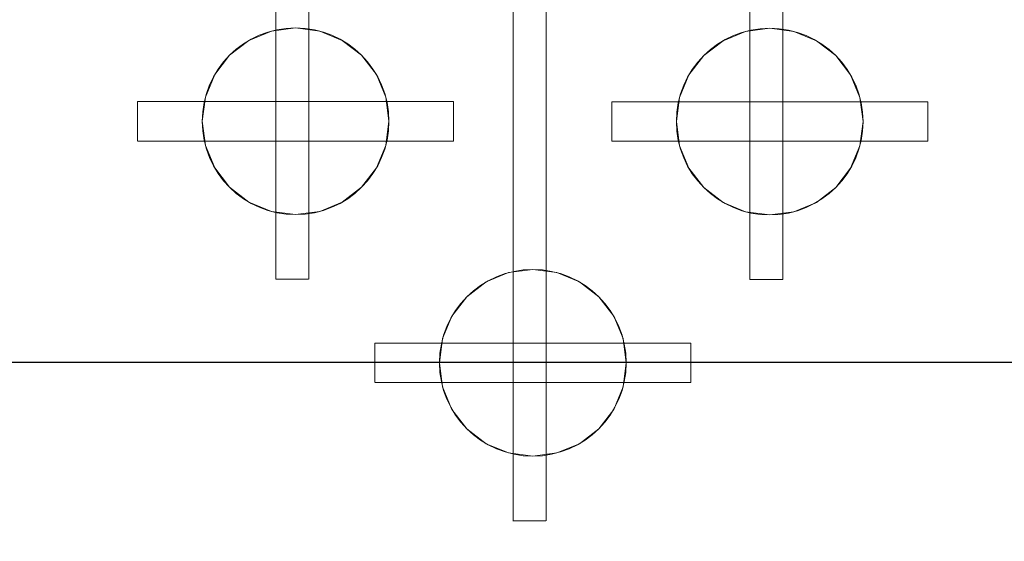
# Model space of a CAD drawing. Units: inches. Extents: x 2696 to 3240, y 1564 to 2310.
# Tile 19 of 76: x 2783.067 to 2792.41, y 1900.004 to 1904.955. Entities that reach past the tile are written whole.
import ezdxf

# ---------------------------------------------------------------- set-up
doc = ezdxf.new("R2010")
doc.units = ezdxf.units.IN
for name, color, linetype, lineweight in [('A-ANNO-DIMS', 3, 'Continuous', 18), ('A-FLOR-FIXT', 8, 'Continuous', 18), ('A-FURN', 251, 'Continuous', 13)]:
    doc.layers.add(name, color=color, linetype=linetype, lineweight=lineweight)
doc.layers.add('FURNITURE', color=250, linetype='Continuous')
doc.styles.add('TIMES NEW', font='times.ttf')
doc.dimstyles.new('Siddhuu', dxfattribs={"dimtxt": 6, "dimasz": 2.5, "dimexe": 1.25, "dimexo": 0.625, "dimtad": 1, "dimdec": 1, "dimlunit": 4, "dimtxsty": 'TIMES NEW', "dimcen": 2.5, "dimclrd": 256, "dimclre": 1, "dimclrt": 7, "dimadec": 0, "dimazin": 0, "dimtfac": 1, "dimtdec": 1, "dimtmove": 0, "dimatfit": 3, "dimfxl": 1, "dimtolj": 1, "dimlwd": -1, "dimarcsym": 0})

# ---------------------------------------------------------------- blocks, each defined once
blk = doc.blocks.new('A$C1af1f523')
at = {"layer": 'A-FURN'}
for p, q in [((-2.9003, 3.9351), (-2.9003, 0.9365)), ((-2.9003, 3.9351, 0.5), (-2.9003, 0.9365, 0.5)), ((-2.9003, 3.9351), (-2.9003, 3.9351, 0.5)), ((-2.5253, 3.9351), (-2.9003, 3.9351)), ((-2.5253, 3.9351, 0.5), (-2.9003, 3.9351, 0.5)), ((-2.5253, 3.9351), (-2.5253, 0.9365)), ((-2.5253, 3.9351, 0.5), (-2.5253, 0.9365, 0.5)), ((-2.5253, 3.9351), (-2.5253, 3.9351, 0.5)), ((-2.9421, 3.2913), (-2.9421, 3.2913, 0.5)), ((-2.7128, 3.3215), (-2.7128, 3.3215, 0.5)), ((-2.4835, 3.2913), (-2.4835, 3.2913, 0.5)), ((-3.1558, 3.2028), (-3.1558, 3.2028, 0.5)), ((-2.2698, 3.2028), (-2.2698, 3.2028, 0.5)), ((-3.3393, 3.062), (-3.3393, 3.062, 0.5)), ((-2.0863, 3.062), (-2.0863, 3.062, 0.5)), ((-3.4801, 2.8785), (-3.4801, 2.8785, 0.5)), ((-1.9455, 2.8785), (-1.9455, 2.8785, 0.5)), ((-3.5686, 2.6648), (-3.5686, 2.6648, 0.5)), ((-1.857, 2.6648), (-1.857, 2.6648, 0.5)), ((0, 2.5605), (-4.2116, 2.5605)), ((0, 2.5605, 0.5), (-4.2116, 2.5605, 0.5)), ((-4.2116, 2.5605), (-4.2116, 2.5605, 0.5)), ((-4.2116, 2.5594), (-4.2116, 2.248)), ((-4.2116, 2.5594, 0.5), (-4.2116, 2.248, 0.5)), ((-4.2116, 2.5594), (-4.2116, 2.5594, 0.5)), ((-3.5988, 2.4355), (-3.5988, 2.4355, 0.5)), ((-1.8268, 2.4355), (-1.8268, 2.4355, 0.5)), ((0, 2.248), (-4.2116, 2.248)), ((0, 2.248, 0.5), (-4.2116, 2.248, 0.5)), ((-4.2116, 2.248), (-4.2116, 2.248, 0.5)), ((-4.2116, 2.248), (-4.2116, 2.2469)), ((-4.2116, 2.248, 0.5), (-4.2116, 2.2469, 0.5)), ((-4.2116, 2.2469), (-4.2116, 2.2469, 0.5)), ((-3.5686, 2.2061), (-3.5686, 2.2061, 0.5)), ((-1.857, 2.2061), (-1.857, 2.2061, 0.5)), ((-3.4801, 1.9924), (-3.4801, 1.9924, 0.5)), ((-1.9455, 1.9924), (-1.9455, 1.9924, 0.5)), ((-3.3393, 1.8089), (-3.3393, 1.8089, 0.5)), ((-2.0863, 1.8089), (-2.0863, 1.8089, 0.5)), ((-4.8156, 1.6871), (-5.1906, 1.6871)), ((-4.8156, 1.6871, 0.5), (-5.1906, 1.6871, 0.5)), ((-5.1906, 1.6871), (-5.1906, 1.6871, 0.5)), ((-5.1906, 1.6871), (-5.1901, -1.3115)), ((-5.1906, 1.6871, 0.5), (-5.1901, -1.3115, 0.5)), ((-4.8156, 1.6871), (-4.8156, 1.6871, 0.5)), ((-4.8156, 1.6871), (-4.8151, -1.3115)), ((-4.8156, 1.6871, 0.5), (-4.8151, -1.3115, 0.5)), ((-3.1558, 1.6681), (-3.1558, 1.6681, 0.5)), ((-2.2698, 1.6681), (-2.2698, 1.6681, 0.5)), ((-2.9421, 1.5796), (-2.9421, 1.5796, 0.5)), ((-2.7128, 1.5494), (-2.7128, 1.5494, 0.5)), ((-2.4835, 1.5796), (-2.4835, 1.5796, 0.5)), ((-5.232, 1.0433), (-5.232, 1.0433, 0.5)), ((-5.0026, 1.0735), (-5.0026, 1.0735, 0.5)), ((-4.7733, 1.0433), (-4.7733, 1.0433, 0.5)), ((-5.4457, 0.9548), (-5.4457, 0.9548, 0.5)), ((-4.5596, 0.9548), (-4.5596, 0.9548, 0.5)), ((-2.9003, 0.9365), (-2.9003, 0.9365, 0.5)), ((-2.5253, 0.9365), (-2.8979, 0.9365)), ((-2.5253, 0.9365, 0.5), (-2.8979, 0.9365, 0.5)), ((-2.8979, 0.9365), (-2.8979, 0.9365, 0.5)), ((-2.5253, 0.9365), (-2.5253, 0.9365, 0.5)), ((-5.6292, 0.814), (-5.6292, 0.814, 0.5)), ((-4.3761, 0.814), (-4.3761, 0.814, 0.5)), ((-5.77, 0.6305), (-5.77, 0.6305, 0.5)), ((-4.2353, 0.6305), (-4.2353, 0.6305, 0.5)), ((-5.8585, 0.4168), (-5.8585, 0.4168, 0.5)), ((-4.1468, 0.4168), (-4.1468, 0.4168, 0.5)), ((0, 0.3125), (-6.5015, 0.3125)), ((0, 0.3125, 0.5), (-6.5015, 0.3125, 0.5)), ((-6.5015, 0.3125), (-6.5015, 0.3125, 0.5)), ((-6.5015, 0.3114), (-6.5015, 0)), ((-6.5015, 0.3114, 0.5), (-6.5015, 0, 0.5)), ((-6.5015, 0.3114), (-6.5015, 0.3114, 0.5)), ((-5.8887, 0.1875), (-5.8887, 0.1875, 0.5)), ((-4.1166, 0.1875), (-4.1166, 0.1875, 0.5)), ((0, 0), (-6.5015, 0)), ((0, 0, 0.5), (-6.5015, 0, 0.5)), ((-6.5015, 0), (-6.5015, 0, 0.5)), ((-6.5015, 0), (-6.5015, -0.0011)), ((-6.5015, 0, 0.5), (-6.5015, -0.0011, 0.5)), ((-6.5015, -0.0011), (-6.5015, -0.0011, 0.5)), ((-5.8585, -0.0418), (-5.8585, -0.0418, 0.5)), ((-4.1468, -0.0418), (-4.1468, -0.0418, 0.5)), ((-5.77, -0.2555), (-5.77, -0.2555, 0.5)), ((-4.2353, -0.2555), (-4.2353, -0.2555, 0.5)), ((-5.6292, -0.439), (-5.6292, -0.439, 0.5)), ((-4.3761, -0.439), (-4.3761, -0.439, 0.5)), ((-5.4457, -0.5798), (-5.4457, -0.5798, 0.5)), ((-4.5596, -0.5798), (-4.5596, -0.5798, 0.5)), ((-2.898, -0.5642), (-2.898, -3.5628)), ((-2.898, -0.5642, 0.5), (-2.898, -3.5628, 0.5)), ((-2.898, -0.5642), (-2.898, -0.5642, 0.5)), ((-2.523, -0.5642), (-2.898, -0.5642)), ((-2.523, -0.5642, 0.5), (-2.898, -0.5642, 0.5)), ((-2.523, -0.5642), (-2.523, -3.5628)), ((-2.523, -0.5642, 0.5), (-2.523, -3.5628, 0.5)), ((-2.523, -0.5642), (-2.523, -0.5642, 0.5)), ((-5.232, -0.6683), (-5.232, -0.6683, 0.5)), ((-5.0026, -0.6985), (-5.0026, -0.6985, 0.5)), ((-4.7733, -0.6683), (-4.7733, -0.6683, 0.5)), ((-2.9398, -1.208), (-2.9398, -1.208, 0.5)), ((-2.7105, -1.1778), (-2.7105, -1.1778, 0.5)), ((-2.4812, -1.208), (-2.4812, -1.208, 0.5)), ((-3.1535, -1.2965), (-3.1535, -1.2965, 0.5)), ((-2.2675, -1.2965), (-2.2675, -1.2965, 0.5)), ((-5.1901, -1.3115), (-5.1901, -1.3115, 0.5)), ((-4.8151, -1.3115), (-5.1878, -1.3115)), ((-4.8151, -1.3115, 0.5), (-5.1878, -1.3115, 0.5)), ((-5.1878, -1.3115), (-5.1878, -1.3115, 0.5)), ((-4.8151, -1.3115), (-4.8151, -1.3115, 0.5)), ((-3.337, -1.4373), (-3.337, -1.4373, 0.5)), ((-2.084, -1.4373), (-2.084, -1.4373, 0.5)), ((-3.4778, -1.6208), (-3.4778, -1.6208, 0.5)), ((-1.9432, -1.6208), (-1.9432, -1.6208, 0.5)), ((-3.5664, -1.8345), (-3.5664, -1.8345, 0.5)), ((-1.8547, -1.8345), (-1.8547, -1.8345, 0.5)), ((0, -1.9388), (-4.2094, -1.9388)), ((0, -1.9388, 0.5), (-4.2094, -1.9388, 0.5)), ((-4.2094, -1.9388), (-4.2094, -1.9388, 0.5)), ((-4.2094, -1.9399), (-4.2094, -2.2513)), ((-4.2094, -1.9399, 0.5), (-4.2094, -2.2513, 0.5)), ((-4.2094, -1.9399), (-4.2094, -1.9399, 0.5)), ((-3.5965, -2.0638), (-3.5965, -2.0638, 0.5)), ((-1.8245, -2.0638), (-1.8245, -2.0638, 0.5)), ((0, -2.2513), (-4.2094, -2.2513)), ((0, -2.2513, 0.5), (-4.2094, -2.2513, 0.5)), ((-4.2094, -2.2513), (-4.2094, -2.2513, 0.5)), ((-4.2094, -2.2513), (-4.2094, -2.2524)), ((-4.2094, -2.2513, 0.5), (-4.2094, -2.2524, 0.5)), ((-4.2094, -2.2524), (-4.2094, -2.2524, 0.5)), ((-3.5664, -2.2931), (-3.5664, -2.2931, 0.5)), ((-1.8547, -2.2931), (-1.8547, -2.2931, 0.5)), ((-3.4778, -2.5068), (-3.4778, -2.5068, 0.5)), ((-1.9432, -2.5068), (-1.9432, -2.5068, 0.5)), ((-3.337, -2.6903), (-3.337, -2.6903, 0.5)), ((-2.084, -2.6903), (-2.084, -2.6903, 0.5)), ((-3.1535, -2.8311), (-3.1535, -2.8311, 0.5)), ((-2.2675, -2.8311), (-2.2675, -2.8311, 0.5)), ((-2.9398, -2.9196), (-2.9398, -2.9196, 0.5)), ((-2.7105, -2.9498), (-2.7105, -2.9498, 0.5)), ((-2.4812, -2.9196), (-2.4812, -2.9196, 0.5)), ((-2.898, -3.5628), (-2.898, -3.5628, 0.5)), ((-2.523, -3.5628), (-2.8956, -3.5628)), ((-2.523, -3.5628, 0.5), (-2.8956, -3.5628, 0.5)), ((-2.8956, -3.5628), (-2.8956, -3.5628, 0.5)), ((-2.523, -3.5628), (-2.523, -3.5628, 0.5))]:
    blk.add_line(p, q, dxfattribs=at)
for centre in [(-2.7128, 2.4355), (-2.7128, 2.4355, 0.5), (-5.0026, 0.1875), (-5.0026, 0.1875, 0.5), (-2.7105, -2.0638), (-2.7105, -2.0638, 0.5)]:
    blk.add_circle(centre, 0.886, dxfattribs=at)
at = {"layer": 'FURNITURE'}
for p, q in [((0, 2.5605), (0, 2.5605, 0.5)), ((0, 2.248), (0, 2.248, 0.5)), ((0, 0.3125), (0, 0.3125, 0.5)), ((0, 0), (0, 0, 0.5)), ((0, -1.9388), (0, -1.9388, 0.5)), ((0, -2.2513), (0, -2.2513, 0.5))]:
    blk.add_line(p, q, dxfattribs=at)
at = {"layer": 'A-FURN'}
mesh = blk.add_polyface(dxfattribs=at)
corners = [(-2.9003, 0.9365, 0.5), (-2.9003, 3.9351), (-2.9003, 0.9365), (-2.9003, 3.9351, 0.5)]
mesh.append_faces([[corners[k] for k in face] for face in [(2, 1, 0), (3, 0, 1)]], dxfattribs={"vtx1": -1})
mesh = blk.add_polyface(dxfattribs=at)
corners = [(-2.5253, 3.9351, 0.5), (-2.9003, 3.9351), (-2.9003, 3.9351, 0.5), (-2.5253, 3.9351)]
mesh.append_faces([[corners[k] for k in face] for face in [(2, 1, 0), (3, 0, 1)]], dxfattribs={"vtx1": -1})
mesh = blk.add_polyface(dxfattribs=at)
corners = [(-2.5253, 0.9365, 0.5), (-2.5253, 3.9351), (-2.5253, 0.9365), (-2.5253, 3.9351, 0.5)]
mesh.append_faces([[corners[k] for k in face] for face in [(2, 1, 0), (3, 0, 1)]], dxfattribs={"vtx1": -1})
mesh = blk.add_polyface(dxfattribs=at)
corners = [(-2.9421, 3.2913), (-3.1558, 3.2028, 0.5), (-3.1558, 3.2028), (-2.9421, 3.2913, 0.5)]
mesh.append_faces([[corners[k] for k in face] for face in [(2, 1, 0), (3, 0, 1)]], dxfattribs={"vtx1": -1})
mesh = blk.add_polyface(dxfattribs=at)
corners = [(-2.7128, 3.3215), (-2.9421, 3.2913, 0.5), (-2.9421, 3.2913), (-2.7128, 3.3215, 0.5)]
mesh.append_faces([[corners[k] for k in face] for face in [(2, 1, 0), (3, 0, 1)]], dxfattribs={"vtx1": -1})
mesh = blk.add_polyface(dxfattribs=at)
corners = [(-2.4835, 3.2913), (-2.7128, 3.3215, 0.5), (-2.7128, 3.3215), (-2.4835, 3.2913, 0.5)]
mesh.append_faces([[corners[k] for k in face] for face in [(2, 1, 0), (3, 0, 1)]], dxfattribs={"vtx1": -1})
mesh = blk.add_polyface(dxfattribs=at)
corners = [(-2.2698, 3.2028), (-2.4835, 3.2913, 0.5), (-2.4835, 3.2913), (-2.2698, 3.2028, 0.5)]
mesh.append_faces([[corners[k] for k in face] for face in [(2, 1, 0), (3, 0, 1)]], dxfattribs={"vtx1": -1})
mesh = blk.add_polyface(dxfattribs=at)
corners = [(-3.1558, 3.2028), (-3.3393, 3.062, 0.5), (-3.3393, 3.062), (-3.1558, 3.2028, 0.5)]
mesh.append_faces([[corners[k] for k in face] for face in [(2, 1, 0), (3, 0, 1)]], dxfattribs={"vtx1": -1})
mesh = blk.add_polyface(dxfattribs=at)
corners = [(-2.0863, 3.062), (-2.2698, 3.2028, 0.5), (-2.2698, 3.2028), (-2.0863, 3.062, 0.5)]
mesh.append_faces([[corners[k] for k in face] for face in [(2, 1, 0), (3, 0, 1)]], dxfattribs={"vtx1": -1})
mesh = blk.add_polyface(dxfattribs=at)
corners = [(-3.3393, 3.062, 0.5), (-3.4801, 2.8785), (-3.3393, 3.062), (-3.4801, 2.8785, 0.5)]
mesh.append_faces([[corners[k] for k in face] for face in [(2, 1, 0), (3, 0, 1)]], dxfattribs={"vtx1": -1})
mesh = blk.add_polyface(dxfattribs=at)
corners = [(-1.9455, 2.8785, 0.5), (-2.0863, 3.062), (-1.9455, 2.8785), (-2.0863, 3.062, 0.5)]
mesh.append_faces([[corners[k] for k in face] for face in [(2, 1, 0), (3, 0, 1)]], dxfattribs={"vtx1": -1})
mesh = blk.add_polyface(dxfattribs=at)
corners = [(-3.4801, 2.8785, 0.5), (-3.5686, 2.6648), (-3.4801, 2.8785), (-3.5686, 2.6648, 0.5)]
mesh.append_faces([[corners[k] for k in face] for face in [(2, 1, 0), (3, 0, 1)]], dxfattribs={"vtx1": -1})
mesh = blk.add_polyface(dxfattribs=at)
corners = [(-1.857, 2.6648, 0.5), (-1.9455, 2.8785), (-1.857, 2.6648), (-1.9455, 2.8785, 0.5)]
mesh.append_faces([[corners[k] for k in face] for face in [(2, 1, 0), (3, 0, 1)]], dxfattribs={"vtx1": -1})
mesh = blk.add_polyface(dxfattribs=at)
corners = [(-3.5686, 2.6648, 0.5), (-3.5988, 2.4355), (-3.5686, 2.6648), (-3.5988, 2.4355, 0.5)]
mesh.append_faces([[corners[k] for k in face] for face in [(2, 1, 0), (3, 0, 1)]], dxfattribs={"vtx1": -1})
mesh = blk.add_polyface(dxfattribs=at)
corners = [(-1.8268, 2.4355, 0.5), (-1.857, 2.6648), (-1.8268, 2.4355), (-1.857, 2.6648, 0.5)]
mesh.append_faces([[corners[k] for k in face] for face in [(2, 1, 0), (3, 0, 1)]], dxfattribs={"vtx1": -1})
mesh = blk.add_polyface(dxfattribs=at)
corners = [(0, 2.5605, 0.5), (-4.2116, 2.5605), (-4.2116, 2.5605, 0.5), (0, 2.5605)]
mesh.append_faces([[corners[k] for k in face] for face in [(2, 1, 0), (3, 0, 1)]], dxfattribs={"vtx1": -1})
mesh = blk.add_polyface(dxfattribs=at)
corners = [(-4.2116, 2.2469, 0.5), (-4.2116, 2.248), (-4.2116, 2.2469), (-4.2116, 2.5594), (-4.2116, 2.5594, 0.5), (-4.2116, 2.248, 0.5)]
mesh.append_faces([[corners[k] for k in face] for face in [(3, 0, 1), (4, 0, 3)]], dxfattribs={"vtx0": -1, "vtx1": -1})
mesh.append_faces([[corners[k] for k in face] for face in [(2, 1, 0), (5, 0, 4)]], dxfattribs={"vtx1": -1})
mesh = blk.add_polyface(dxfattribs=at)
corners = [(-3.5988, 2.4355, 0.5), (-3.5686, 2.2061), (-3.5988, 2.4355), (-3.5686, 2.2061, 0.5)]
mesh.append_faces([[corners[k] for k in face] for face in [(2, 1, 0), (3, 0, 1)]], dxfattribs={"vtx1": -1})
mesh = blk.add_polyface(dxfattribs=at)
corners = [(-1.857, 2.2061, 0.5), (-1.8268, 2.4355), (-1.857, 2.2061), (-1.8268, 2.4355, 0.5)]
mesh.append_faces([[corners[k] for k in face] for face in [(2, 1, 0), (3, 0, 1)]], dxfattribs={"vtx1": -1})
mesh = blk.add_polyface(dxfattribs=at)
corners = [(0, 2.248, 0.5), (-4.2116, 2.248), (-4.2116, 2.248, 0.5), (0, 2.248)]
mesh.append_faces([[corners[k] for k in face] for face in [(2, 1, 0), (3, 0, 1)]], dxfattribs={"vtx1": -1})
mesh = blk.add_polyface(dxfattribs=at)
corners = [(-3.5686, 2.2061, 0.5), (-3.4801, 1.9924), (-3.5686, 2.2061), (-3.4801, 1.9924, 0.5)]
mesh.append_faces([[corners[k] for k in face] for face in [(2, 1, 0), (3, 0, 1)]], dxfattribs={"vtx1": -1})
mesh = blk.add_polyface(dxfattribs=at)
corners = [(-1.9455, 1.9924, 0.5), (-1.857, 2.2061), (-1.9455, 1.9924), (-1.857, 2.2061, 0.5)]
mesh.append_faces([[corners[k] for k in face] for face in [(2, 1, 0), (3, 0, 1)]], dxfattribs={"vtx1": -1})
mesh = blk.add_polyface(dxfattribs=at)
corners = [(-3.4801, 1.9924, 0.5), (-3.3393, 1.8089), (-3.4801, 1.9924), (-3.3393, 1.8089, 0.5)]
mesh.append_faces([[corners[k] for k in face] for face in [(2, 1, 0), (3, 0, 1)]], dxfattribs={"vtx1": -1})
mesh = blk.add_polyface(dxfattribs=at)
corners = [(-2.0863, 1.8089, 0.5), (-1.9455, 1.9924), (-2.0863, 1.8089), (-1.9455, 1.9924, 0.5)]
mesh.append_faces([[corners[k] for k in face] for face in [(2, 1, 0), (3, 0, 1)]], dxfattribs={"vtx1": -1})
mesh = blk.add_polyface(dxfattribs=at)
corners = [(-3.1558, 1.6681, 0.5), (-3.3393, 1.8089), (-3.3393, 1.8089, 0.5), (-3.1558, 1.6681)]
mesh.append_faces([[corners[k] for k in face] for face in [(2, 1, 0), (3, 0, 1)]], dxfattribs={"vtx1": -1})
mesh = blk.add_polyface(dxfattribs=at)
corners = [(-2.0863, 1.8089, 0.5), (-2.2698, 1.6681), (-2.2698, 1.6681, 0.5), (-2.0863, 1.8089)]
mesh.append_faces([[corners[k] for k in face] for face in [(2, 1, 0), (3, 0, 1)]], dxfattribs={"vtx1": -1})
mesh = blk.add_polyface(dxfattribs=at)
corners = [(-4.8156, 1.6871, 0.5), (-5.1906, 1.6871), (-5.1906, 1.6871, 0.5), (-4.8156, 1.6871)]
mesh.append_faces([[corners[k] for k in face] for face in [(2, 1, 0), (3, 0, 1)]], dxfattribs={"vtx1": -1})
mesh = blk.add_polyface(dxfattribs=at)
corners = [(-5.1901, -1.3115, 0.5), (-5.1906, 1.6871), (-5.1901, -1.3115), (-5.1906, 1.6871, 0.5)]
mesh.append_faces([[corners[k] for k in face] for face in [(2, 1, 0), (3, 0, 1)]], dxfattribs={"vtx1": -1})
mesh = blk.add_polyface(dxfattribs=at)
corners = [(-4.8151, -1.3115, 0.5), (-4.8156, 1.6871), (-4.8151, -1.3115), (-4.8156, 1.6871, 0.5)]
mesh.append_faces([[corners[k] for k in face] for face in [(2, 1, 0), (3, 0, 1)]], dxfattribs={"vtx1": -1})
mesh = blk.add_polyface(dxfattribs=at)
corners = [(-2.9421, 1.5796, 0.5), (-3.1558, 1.6681), (-3.1558, 1.6681, 0.5), (-2.9421, 1.5796)]
mesh.append_faces([[corners[k] for k in face] for face in [(2, 1, 0), (3, 0, 1)]], dxfattribs={"vtx1": -1})
mesh = blk.add_polyface(dxfattribs=at)
corners = [(-2.2698, 1.6681, 0.5), (-2.4835, 1.5796), (-2.4835, 1.5796, 0.5), (-2.2698, 1.6681)]
mesh.append_faces([[corners[k] for k in face] for face in [(2, 1, 0), (3, 0, 1)]], dxfattribs={"vtx1": -1})
mesh = blk.add_polyface(dxfattribs=at)
corners = [(-2.7128, 1.5494, 0.5), (-2.9421, 1.5796), (-2.9421, 1.5796, 0.5), (-2.7128, 1.5494)]
mesh.append_faces([[corners[k] for k in face] for face in [(2, 1, 0), (3, 0, 1)]], dxfattribs={"vtx1": -1})
mesh = blk.add_polyface(dxfattribs=at)
corners = [(-2.4835, 1.5796, 0.5), (-2.7128, 1.5494), (-2.7128, 1.5494, 0.5), (-2.4835, 1.5796)]
mesh.append_faces([[corners[k] for k in face] for face in [(2, 1, 0), (3, 0, 1)]], dxfattribs={"vtx1": -1})
mesh = blk.add_polyface(dxfattribs=at)
corners = [(-5.232, 1.0433), (-5.4457, 0.9548, 0.5), (-5.4457, 0.9548), (-5.232, 1.0433, 0.5)]
mesh.append_faces([[corners[k] for k in face] for face in [(2, 1, 0), (3, 0, 1)]], dxfattribs={"vtx1": -1})
mesh = blk.add_polyface(dxfattribs=at)
corners = [(-5.0026, 1.0735), (-5.232, 1.0433, 0.5), (-5.232, 1.0433), (-5.0026, 1.0735, 0.5)]
mesh.append_faces([[corners[k] for k in face] for face in [(2, 1, 0), (3, 0, 1)]], dxfattribs={"vtx1": -1})
mesh = blk.add_polyface(dxfattribs=at)
corners = [(-4.7733, 1.0433), (-5.0026, 1.0735, 0.5), (-5.0026, 1.0735), (-4.7733, 1.0433, 0.5)]
mesh.append_faces([[corners[k] for k in face] for face in [(2, 1, 0), (3, 0, 1)]], dxfattribs={"vtx1": -1})
mesh = blk.add_polyface(dxfattribs=at)
corners = [(-4.5596, 0.9548), (-4.7733, 1.0433, 0.5), (-4.7733, 1.0433), (-4.5596, 0.9548, 0.5)]
mesh.append_faces([[corners[k] for k in face] for face in [(2, 1, 0), (3, 0, 1)]], dxfattribs={"vtx1": -1})
mesh = blk.add_polyface(dxfattribs=at)
corners = [(-5.4457, 0.9548), (-5.6292, 0.814, 0.5), (-5.6292, 0.814), (-5.4457, 0.9548, 0.5)]
mesh.append_faces([[corners[k] for k in face] for face in [(2, 1, 0), (3, 0, 1)]], dxfattribs={"vtx1": -1})
mesh = blk.add_polyface(dxfattribs=at)
corners = [(-4.3761, 0.814), (-4.5596, 0.9548, 0.5), (-4.5596, 0.9548), (-4.3761, 0.814, 0.5)]
mesh.append_faces([[corners[k] for k in face] for face in [(2, 1, 0), (3, 0, 1)]], dxfattribs={"vtx1": -1})
mesh = blk.add_polyface(dxfattribs=at)
corners = [(-2.5253, 0.9365, 0.5), (-2.8979, 0.9365), (-2.8979, 0.9365, 0.5), (-2.5253, 0.9365)]
mesh.append_faces([[corners[k] for k in face] for face in [(2, 1, 0), (3, 0, 1)]], dxfattribs={"vtx1": -1})
mesh = blk.add_polyface(dxfattribs=at)
corners = [(-5.6292, 0.814, 0.5), (-5.77, 0.6305), (-5.6292, 0.814), (-5.77, 0.6305, 0.5)]
mesh.append_faces([[corners[k] for k in face] for face in [(2, 1, 0), (3, 0, 1)]], dxfattribs={"vtx1": -1})
mesh = blk.add_polyface(dxfattribs=at)
corners = [(-4.2353, 0.6305, 0.5), (-4.3761, 0.814), (-4.2353, 0.6305), (-4.3761, 0.814, 0.5)]
mesh.append_faces([[corners[k] for k in face] for face in [(2, 1, 0), (3, 0, 1)]], dxfattribs={"vtx1": -1})
mesh = blk.add_polyface(dxfattribs=at)
corners = [(-5.77, 0.6305, 0.5), (-5.8585, 0.4168), (-5.77, 0.6305), (-5.8585, 0.4168, 0.5)]
mesh.append_faces([[corners[k] for k in face] for face in [(2, 1, 0), (3, 0, 1)]], dxfattribs={"vtx1": -1})
mesh = blk.add_polyface(dxfattribs=at)
corners = [(-4.1468, 0.4168, 0.5), (-4.2353, 0.6305), (-4.1468, 0.4168), (-4.2353, 0.6305, 0.5)]
mesh.append_faces([[corners[k] for k in face] for face in [(2, 1, 0), (3, 0, 1)]], dxfattribs={"vtx1": -1})
mesh = blk.add_polyface(dxfattribs=at)
corners = [(-5.8585, 0.4168, 0.5), (-5.8887, 0.1875), (-5.8585, 0.4168), (-5.8887, 0.1875, 0.5)]
mesh.append_faces([[corners[k] for k in face] for face in [(2, 1, 0), (3, 0, 1)]], dxfattribs={"vtx1": -1})
mesh = blk.add_polyface(dxfattribs=at)
corners = [(-4.1166, 0.1875, 0.5), (-4.1468, 0.4168), (-4.1166, 0.1875), (-4.1468, 0.4168, 0.5)]
mesh.append_faces([[corners[k] for k in face] for face in [(2, 1, 0), (3, 0, 1)]], dxfattribs={"vtx1": -1})
mesh = blk.add_polyface(dxfattribs=at)
corners = [(0, 0.3125, 0.5), (-6.5015, 0.3125), (-6.5015, 0.3125, 0.5), (0, 0.3125)]
mesh.append_faces([[corners[k] for k in face] for face in [(2, 1, 0), (3, 0, 1)]], dxfattribs={"vtx1": -1})
mesh = blk.add_polyface(dxfattribs=at)
corners = [(-6.5015, -0.0011, 0.5), (-6.5015, 0), (-6.5015, -0.0011), (-6.5015, 0.3114), (-6.5015, 0.3114, 0.5), (-6.5015, 0, 0.5)]
mesh.append_faces([[corners[k] for k in face] for face in [(3, 0, 1), (4, 0, 3)]], dxfattribs={"vtx0": -1, "vtx1": -1})
mesh.append_faces([[corners[k] for k in face] for face in [(2, 1, 0), (5, 0, 4)]], dxfattribs={"vtx1": -1})
mesh = blk.add_polyface(dxfattribs=at)
corners = [(-5.8887, 0.1875, 0.5), (-5.8585, -0.0418), (-5.8887, 0.1875), (-5.8585, -0.0418, 0.5)]
mesh.append_faces([[corners[k] for k in face] for face in [(2, 1, 0), (3, 0, 1)]], dxfattribs={"vtx1": -1})
mesh = blk.add_polyface(dxfattribs=at)
corners = [(-4.1468, -0.0418, 0.5), (-4.1166, 0.1875), (-4.1468, -0.0418), (-4.1166, 0.1875, 0.5)]
mesh.append_faces([[corners[k] for k in face] for face in [(2, 1, 0), (3, 0, 1)]], dxfattribs={"vtx1": -1})
mesh = blk.add_polyface(dxfattribs=at)
corners = [(0, 0, 0.5), (-6.5015, 0), (-6.5015, 0, 0.5), (0, 0)]
mesh.append_faces([[corners[k] for k in face] for face in [(2, 1, 0), (3, 0, 1)]], dxfattribs={"vtx1": -1})
mesh = blk.add_polyface(dxfattribs=at)
corners = [(-5.8585, -0.0418, 0.5), (-5.77, -0.2555), (-5.8585, -0.0418), (-5.77, -0.2555, 0.5)]
mesh.append_faces([[corners[k] for k in face] for face in [(2, 1, 0), (3, 0, 1)]], dxfattribs={"vtx1": -1})
mesh = blk.add_polyface(dxfattribs=at)
corners = [(-4.2353, -0.2555, 0.5), (-4.1468, -0.0418), (-4.2353, -0.2555), (-4.1468, -0.0418, 0.5)]
mesh.append_faces([[corners[k] for k in face] for face in [(2, 1, 0), (3, 0, 1)]], dxfattribs={"vtx1": -1})
mesh = blk.add_polyface(dxfattribs=at)
corners = [(-5.77, -0.2555, 0.5), (-5.6292, -0.439), (-5.77, -0.2555), (-5.6292, -0.439, 0.5)]
mesh.append_faces([[corners[k] for k in face] for face in [(2, 1, 0), (3, 0, 1)]], dxfattribs={"vtx1": -1})
mesh = blk.add_polyface(dxfattribs=at)
corners = [(-4.3761, -0.439, 0.5), (-4.2353, -0.2555), (-4.3761, -0.439), (-4.2353, -0.2555, 0.5)]
mesh.append_faces([[corners[k] for k in face] for face in [(2, 1, 0), (3, 0, 1)]], dxfattribs={"vtx1": -1})
mesh = blk.add_polyface(dxfattribs=at)
corners = [(-5.4457, -0.5798, 0.5), (-5.6292, -0.439), (-5.6292, -0.439, 0.5), (-5.4457, -0.5798)]
mesh.append_faces([[corners[k] for k in face] for face in [(2, 1, 0), (3, 0, 1)]], dxfattribs={"vtx1": -1})
mesh = blk.add_polyface(dxfattribs=at)
corners = [(-4.3761, -0.439, 0.5), (-4.5596, -0.5798), (-4.5596, -0.5798, 0.5), (-4.3761, -0.439)]
mesh.append_faces([[corners[k] for k in face] for face in [(2, 1, 0), (3, 0, 1)]], dxfattribs={"vtx1": -1})
mesh = blk.add_polyface(dxfattribs=at)
corners = [(-5.232, -0.6683, 0.5), (-5.4457, -0.5798), (-5.4457, -0.5798, 0.5), (-5.232, -0.6683)]
mesh.append_faces([[corners[k] for k in face] for face in [(2, 1, 0), (3, 0, 1)]], dxfattribs={"vtx1": -1})
mesh = blk.add_polyface(dxfattribs=at)
corners = [(-4.5596, -0.5798, 0.5), (-4.7733, -0.6683), (-4.7733, -0.6683, 0.5), (-4.5596, -0.5798)]
mesh.append_faces([[corners[k] for k in face] for face in [(2, 1, 0), (3, 0, 1)]], dxfattribs={"vtx1": -1})
mesh = blk.add_polyface(dxfattribs=at)
corners = [(-2.898, -3.5628, 0.5), (-2.898, -0.5642), (-2.898, -3.5628), (-2.898, -0.5642, 0.5)]
mesh.append_faces([[corners[k] for k in face] for face in [(2, 1, 0), (3, 0, 1)]], dxfattribs={"vtx1": -1})
mesh = blk.add_polyface(dxfattribs=at)
corners = [(-2.523, -0.5642, 0.5), (-2.898, -0.5642), (-2.898, -0.5642, 0.5), (-2.523, -0.5642)]
mesh.append_faces([[corners[k] for k in face] for face in [(2, 1, 0), (3, 0, 1)]], dxfattribs={"vtx1": -1})
mesh = blk.add_polyface(dxfattribs=at)
corners = [(-2.523, -3.5628, 0.5), (-2.523, -0.5642), (-2.523, -3.5628), (-2.523, -0.5642, 0.5)]
mesh.append_faces([[corners[k] for k in face] for face in [(2, 1, 0), (3, 0, 1)]], dxfattribs={"vtx1": -1})
mesh = blk.add_polyface(dxfattribs=at)
corners = [(-5.0026, -0.6985, 0.5), (-5.232, -0.6683), (-5.232, -0.6683, 0.5), (-5.0026, -0.6985)]
mesh.append_faces([[corners[k] for k in face] for face in [(2, 1, 0), (3, 0, 1)]], dxfattribs={"vtx1": -1})
mesh = blk.add_polyface(dxfattribs=at)
corners = [(-4.7733, -0.6683, 0.5), (-5.0026, -0.6985), (-5.0026, -0.6985, 0.5), (-4.7733, -0.6683)]
mesh.append_faces([[corners[k] for k in face] for face in [(2, 1, 0), (3, 0, 1)]], dxfattribs={"vtx1": -1})
mesh = blk.add_polyface(dxfattribs=at)
corners = [(-2.9398, -1.208), (-3.1535, -1.2965, 0.5), (-3.1535, -1.2965), (-2.9398, -1.208, 0.5)]
mesh.append_faces([[corners[k] for k in face] for face in [(2, 1, 0), (3, 0, 1)]], dxfattribs={"vtx1": -1})
mesh = blk.add_polyface(dxfattribs=at)
corners = [(-2.7105, -1.1778), (-2.9398, -1.208, 0.5), (-2.9398, -1.208), (-2.7105, -1.1778, 0.5)]
mesh.append_faces([[corners[k] for k in face] for face in [(2, 1, 0), (3, 0, 1)]], dxfattribs={"vtx1": -1})
mesh = blk.add_polyface(dxfattribs=at)
corners = [(-2.4812, -1.208), (-2.7105, -1.1778, 0.5), (-2.7105, -1.1778), (-2.4812, -1.208, 0.5)]
mesh.append_faces([[corners[k] for k in face] for face in [(2, 1, 0), (3, 0, 1)]], dxfattribs={"vtx1": -1})
mesh = blk.add_polyface(dxfattribs=at)
corners = [(-2.2675, -1.2965), (-2.4812, -1.208, 0.5), (-2.4812, -1.208), (-2.2675, -1.2965, 0.5)]
mesh.append_faces([[corners[k] for k in face] for face in [(2, 1, 0), (3, 0, 1)]], dxfattribs={"vtx1": -1})
mesh = blk.add_polyface(dxfattribs=at)
corners = [(-3.1535, -1.2965), (-3.337, -1.4373, 0.5), (-3.337, -1.4373), (-3.1535, -1.2965, 0.5)]
mesh.append_faces([[corners[k] for k in face] for face in [(2, 1, 0), (3, 0, 1)]], dxfattribs={"vtx1": -1})
mesh = blk.add_polyface(dxfattribs=at)
corners = [(-2.084, -1.4373), (-2.2675, -1.2965, 0.5), (-2.2675, -1.2965), (-2.084, -1.4373, 0.5)]
mesh.append_faces([[corners[k] for k in face] for face in [(2, 1, 0), (3, 0, 1)]], dxfattribs={"vtx1": -1})
mesh = blk.add_polyface(dxfattribs=at)
corners = [(-4.8151, -1.3115, 0.5), (-5.1878, -1.3115), (-5.1878, -1.3115, 0.5), (-4.8151, -1.3115)]
mesh.append_faces([[corners[k] for k in face] for face in [(2, 1, 0), (3, 0, 1)]], dxfattribs={"vtx1": -1})
mesh = blk.add_polyface(dxfattribs=at)
corners = [(-3.337, -1.4373, 0.5), (-3.4778, -1.6208), (-3.337, -1.4373), (-3.4778, -1.6208, 0.5)]
mesh.append_faces([[corners[k] for k in face] for face in [(2, 1, 0), (3, 0, 1)]], dxfattribs={"vtx1": -1})
mesh = blk.add_polyface(dxfattribs=at)
corners = [(-1.9432, -1.6208, 0.5), (-2.084, -1.4373), (-1.9432, -1.6208), (-2.084, -1.4373, 0.5)]
mesh.append_faces([[corners[k] for k in face] for face in [(2, 1, 0), (3, 0, 1)]], dxfattribs={"vtx1": -1})
mesh = blk.add_polyface(dxfattribs=at)
corners = [(-3.4778, -1.6208, 0.5), (-3.5664, -1.8345), (-3.4778, -1.6208), (-3.5664, -1.8345, 0.5)]
mesh.append_faces([[corners[k] for k in face] for face in [(2, 1, 0), (3, 0, 1)]], dxfattribs={"vtx1": -1})
mesh = blk.add_polyface(dxfattribs=at)
corners = [(-1.8547, -1.8345, 0.5), (-1.9432, -1.6208), (-1.8547, -1.8345), (-1.9432, -1.6208, 0.5)]
mesh.append_faces([[corners[k] for k in face] for face in [(2, 1, 0), (3, 0, 1)]], dxfattribs={"vtx1": -1})
mesh = blk.add_polyface(dxfattribs=at)
corners = [(-3.5664, -1.8345, 0.5), (-3.5965, -2.0638), (-3.5664, -1.8345), (-3.5965, -2.0638, 0.5)]
mesh.append_faces([[corners[k] for k in face] for face in [(2, 1, 0), (3, 0, 1)]], dxfattribs={"vtx1": -1})
mesh = blk.add_polyface(dxfattribs=at)
corners = [(-1.8245, -2.0638, 0.5), (-1.8547, -1.8345), (-1.8245, -2.0638), (-1.8547, -1.8345, 0.5)]
mesh.append_faces([[corners[k] for k in face] for face in [(2, 1, 0), (3, 0, 1)]], dxfattribs={"vtx1": -1})
mesh = blk.add_polyface(dxfattribs=at)
corners = [(0, -1.9388, 0.5), (-4.2094, -1.9388), (-4.2094, -1.9388, 0.5), (0, -1.9388)]
mesh.append_faces([[corners[k] for k in face] for face in [(2, 1, 0), (3, 0, 1)]], dxfattribs={"vtx1": -1})
mesh = blk.add_polyface(dxfattribs=at)
corners = [(-4.2094, -2.2524, 0.5), (-4.2094, -2.2513), (-4.2094, -2.2524), (-4.2094, -1.9399), (-4.2094, -1.9399, 0.5), (-4.2094, -2.2513, 0.5)]
mesh.append_faces([[corners[k] for k in face] for face in [(3, 0, 1), (4, 0, 3)]], dxfattribs={"vtx0": -1, "vtx1": -1})
mesh.append_faces([[corners[k] for k in face] for face in [(2, 1, 0), (5, 0, 4)]], dxfattribs={"vtx1": -1})
mesh = blk.add_polyface(dxfattribs=at)
corners = [(-3.5965, -2.0638, 0.5), (-3.5664, -2.2931), (-3.5965, -2.0638), (-3.5664, -2.2931, 0.5)]
mesh.append_faces([[corners[k] for k in face] for face in [(2, 1, 0), (3, 0, 1)]], dxfattribs={"vtx1": -1})
mesh = blk.add_polyface(dxfattribs=at)
corners = [(-1.8547, -2.2931, 0.5), (-1.8245, -2.0638), (-1.8547, -2.2931), (-1.8245, -2.0638, 0.5)]
mesh.append_faces([[corners[k] for k in face] for face in [(2, 1, 0), (3, 0, 1)]], dxfattribs={"vtx1": -1})
mesh = blk.add_polyface(dxfattribs=at)
corners = [(0, -2.2513, 0.5), (-4.2094, -2.2513), (-4.2094, -2.2513, 0.5), (0, -2.2513)]
mesh.append_faces([[corners[k] for k in face] for face in [(2, 1, 0), (3, 0, 1)]], dxfattribs={"vtx1": -1})
mesh = blk.add_polyface(dxfattribs=at)
corners = [(-3.5664, -2.2931, 0.5), (-3.4778, -2.5068), (-3.5664, -2.2931), (-3.4778, -2.5068, 0.5)]
mesh.append_faces([[corners[k] for k in face] for face in [(2, 1, 0), (3, 0, 1)]], dxfattribs={"vtx1": -1})
mesh = blk.add_polyface(dxfattribs=at)
corners = [(-1.9432, -2.5068, 0.5), (-1.8547, -2.2931), (-1.9432, -2.5068), (-1.8547, -2.2931, 0.5)]
mesh.append_faces([[corners[k] for k in face] for face in [(2, 1, 0), (3, 0, 1)]], dxfattribs={"vtx1": -1})
mesh = blk.add_polyface(dxfattribs=at)
corners = [(-3.4778, -2.5068, 0.5), (-3.337, -2.6903), (-3.4778, -2.5068), (-3.337, -2.6903, 0.5)]
mesh.append_faces([[corners[k] for k in face] for face in [(2, 1, 0), (3, 0, 1)]], dxfattribs={"vtx1": -1})
mesh = blk.add_polyface(dxfattribs=at)
corners = [(-2.084, -2.6903, 0.5), (-1.9432, -2.5068), (-2.084, -2.6903), (-1.9432, -2.5068, 0.5)]
mesh.append_faces([[corners[k] for k in face] for face in [(2, 1, 0), (3, 0, 1)]], dxfattribs={"vtx1": -1})
mesh = blk.add_polyface(dxfattribs=at)
corners = [(-3.1535, -2.8311, 0.5), (-3.337, -2.6903), (-3.337, -2.6903, 0.5), (-3.1535, -2.8311)]
mesh.append_faces([[corners[k] for k in face] for face in [(2, 1, 0), (3, 0, 1)]], dxfattribs={"vtx1": -1})
mesh = blk.add_polyface(dxfattribs=at)
corners = [(-2.084, -2.6903, 0.5), (-2.2675, -2.8311), (-2.2675, -2.8311, 0.5), (-2.084, -2.6903)]
mesh.append_faces([[corners[k] for k in face] for face in [(2, 1, 0), (3, 0, 1)]], dxfattribs={"vtx1": -1})
mesh = blk.add_polyface(dxfattribs=at)
corners = [(-2.9398, -2.9196, 0.5), (-3.1535, -2.8311), (-3.1535, -2.8311, 0.5), (-2.9398, -2.9196)]
mesh.append_faces([[corners[k] for k in face] for face in [(2, 1, 0), (3, 0, 1)]], dxfattribs={"vtx1": -1})
mesh = blk.add_polyface(dxfattribs=at)
corners = [(-2.2675, -2.8311, 0.5), (-2.4812, -2.9196), (-2.4812, -2.9196, 0.5), (-2.2675, -2.8311)]
mesh.append_faces([[corners[k] for k in face] for face in [(2, 1, 0), (3, 0, 1)]], dxfattribs={"vtx1": -1})
mesh = blk.add_polyface(dxfattribs=at)
corners = [(-2.7105, -2.9498, 0.5), (-2.9398, -2.9196), (-2.9398, -2.9196, 0.5), (-2.7105, -2.9498)]
mesh.append_faces([[corners[k] for k in face] for face in [(2, 1, 0), (3, 0, 1)]], dxfattribs={"vtx1": -1})
mesh = blk.add_polyface(dxfattribs=at)
corners = [(-2.4812, -2.9196, 0.5), (-2.7105, -2.9498), (-2.7105, -2.9498, 0.5), (-2.4812, -2.9196)]
mesh.append_faces([[corners[k] for k in face] for face in [(2, 1, 0), (3, 0, 1)]], dxfattribs={"vtx1": -1})
mesh = blk.add_polyface(dxfattribs=at)
corners = [(-2.523, -3.5628, 0.5), (-2.8956, -3.5628), (-2.8956, -3.5628, 0.5), (-2.523, -3.5628)]
mesh.append_faces([[corners[k] for k in face] for face in [(2, 1, 0), (3, 0, 1)]], dxfattribs={"vtx1": -1})
blk = doc.blocks.new('*D55')
at = {"layer": 'A-ANNO-DIMS', "color": 1, "lineweight": -2, "transparency": 16777216}
for p, q in [((3189.9864, 1980.2011), (2709.3614, 1980.2011)), ((3189.9864, 1893.2011), (2709.3614, 1893.2011))]:
    blk.add_line(p, q, dxfattribs=at)
at = {"layer": 'A-ANNO-DIMS', "transparency": 16777216}
blk.add_line((2710.6114, 1895.7011), (2710.6114, 1977.7011), dxfattribs=at)
for points in [[(2710.1947, 1977.7011), (2711.0281, 1977.7011), (2710.6114, 1980.2011)], [(2710.1947, 1895.7011), (2711.0281, 1895.7011), (2710.6114, 1893.2011)]]:
    blk.add_solid(points, dxfattribs=at)
at = {"layer": 'Defpoints', "color": 0, "transparency": 16777216}
for p in [(2710.6114, 1980.2011), (3190.6114, 1980.2011), (3190.6114, 1893.2011)]:
    blk.add_point(p, dxfattribs=at)
at = {"layer": 'A-ANNO-DIMS', "color": 7, "transparency": 16777216, "insert": (2706.9258, 1936.7011), "char_height": 6, "attachment_point": 5, "rotation": 90, "style": 'TIMES NEW'}
blk.add_mtext('\\A1;7\'-3"', dxfattribs=at)
blk = doc.blocks.new('*D57')
at = {"layer": 'A-ANNO-DIMS', "color": 1, "lineweight": -2, "transparency": 16777216}
for p, q in [((2754.6114, 2018.5761), (2754.6114, 1568.9511)), ((2956.7088, 2018.5761), (2956.7088, 1568.9511))]:
    blk.add_line(p, q, dxfattribs=at)
at = {"layer": 'A-ANNO-DIMS', "transparency": 16777216}
blk.add_line((2757.1114, 1570.2011), (2954.2088, 1570.2011), dxfattribs=at)
for points in [[(2757.1114, 1570.6178), (2757.1114, 1569.7844), (2754.6114, 1570.2011)], [(2954.2088, 1570.6178), (2954.2088, 1569.7844), (2956.7088, 1570.2011)]]:
    blk.add_solid(points, dxfattribs=at)
at = {"layer": 'Defpoints', "color": 0, "transparency": 16777216}
for p in [(2754.6114, 2019.2011), (2956.7088, 2019.2011), (2956.7088, 1570.2011)]:
    blk.add_point(p, dxfattribs=at)
at = {"layer": 'A-ANNO-DIMS', "color": 7, "transparency": 16777216, "insert": (2855.6601, 1573.878), "char_height": 6, "attachment_point": 5, "style": 'TIMES NEW'}
blk.add_mtext('\\A1;16\'-10"', dxfattribs=at)
blk = doc.blocks.new('*D78')
at = {"layer": 'A-ANNO-DIMS', "transparency": 16777216}
for p, q in [((2710.6114, 1901.7011), (2710.6114, 1935.1007)), ((2710.6114, 1895.7011), (2710.6114, 1899.2011))]:
    blk.add_line(p, q, dxfattribs=at)
at = {"layer": 'A-ANNO-DIMS', "color": 1, "lineweight": -2, "transparency": 16777216}
for p, q in [((3189.9864, 1901.7011), (2709.3614, 1901.7011)), ((3189.9864, 1893.2011), (2709.3614, 1893.2011))]:
    blk.add_line(p, q, dxfattribs=at)
at = {"layer": 'A-ANNO-DIMS', "transparency": 16777216}
for points in [[(2710.1947, 1899.2011), (2711.0281, 1899.2011), (2710.6114, 1901.7011)], [(2710.1947, 1895.7011), (2711.0281, 1895.7011), (2710.6114, 1893.2011)]]:
    blk.add_solid(points, dxfattribs=at)
at = {"layer": 'Defpoints', "color": 0, "transparency": 16777216}
for p in [(2710.6114, 1901.7011), (3190.6114, 1901.7011), (3190.6114, 1893.2011)]:
    blk.add_point(p, dxfattribs=at)
at = {"layer": 'A-ANNO-DIMS', "color": 7, "transparency": 16777216, "insert": (2706.8501, 1919.6509), "char_height": 6, "attachment_point": 5, "rotation": 90, "style": 'TIMES NEW'}
blk.add_mtext('\\A1;0\'-8 1/2"', dxfattribs=at)

msp = doc.modelspace()

# ---------------------------------------------------------------- block references
at = {"layer": 'A-FLOR-FIXT', "xscale": -1, "rotation": 270}
msp.add_blockref('A$C1af1f523', (2787.7487, 1906.7011), dxfattribs=at)

# ---------------------------------------------------------------- dimensions: what is measured, and where the dimension line sits
at = {"layer": 'A-ANNO-DIMS'}
dim = msp.add_linear_dim(base=(2956.7088, 1570.2011), p1=(2754.6114, 2019.2011), p2=(2956.7088, 2019.2011), dimstyle='Siddhuu', override={"dimdec": 1, "dimlfac": 1, "dimrnd": 0, "dimzin": 1, "dimdsep": 46, "dimlunit": 4, "dimfrac": 2}, dxfattribs=at)
dim.commit()
dim.dimension.update_dxf_attribs({"geometry": '*D57', "text_midpoint": (2855.6601, 1573.878)})
for base, p2, picture, middle in [((2710.6114, 1980.2011), (3190.6114, 1980.2011), '*D55', (2706.9258, 1936.7011)), ((2710.6114, 1901.7011), (3190.6114, 1901.7011), '*D78', (2706.8501, 1919.6509))]:
    dim = msp.add_linear_dim(base=base, p1=(3190.6114, 1893.2011), p2=p2, angle=90, dimstyle='Siddhuu', override={"dimdec": 1, "dimlfac": 1, "dimrnd": 0, "dimzin": 1, "dimdsep": 46, "dimlunit": 4, "dimfrac": 2}, dxfattribs=at)
    dim.commit()
    dim.dimension.update_dxf_attribs({"geometry": picture, "text_midpoint": middle})

doc.saveas('drawing.dxf')
